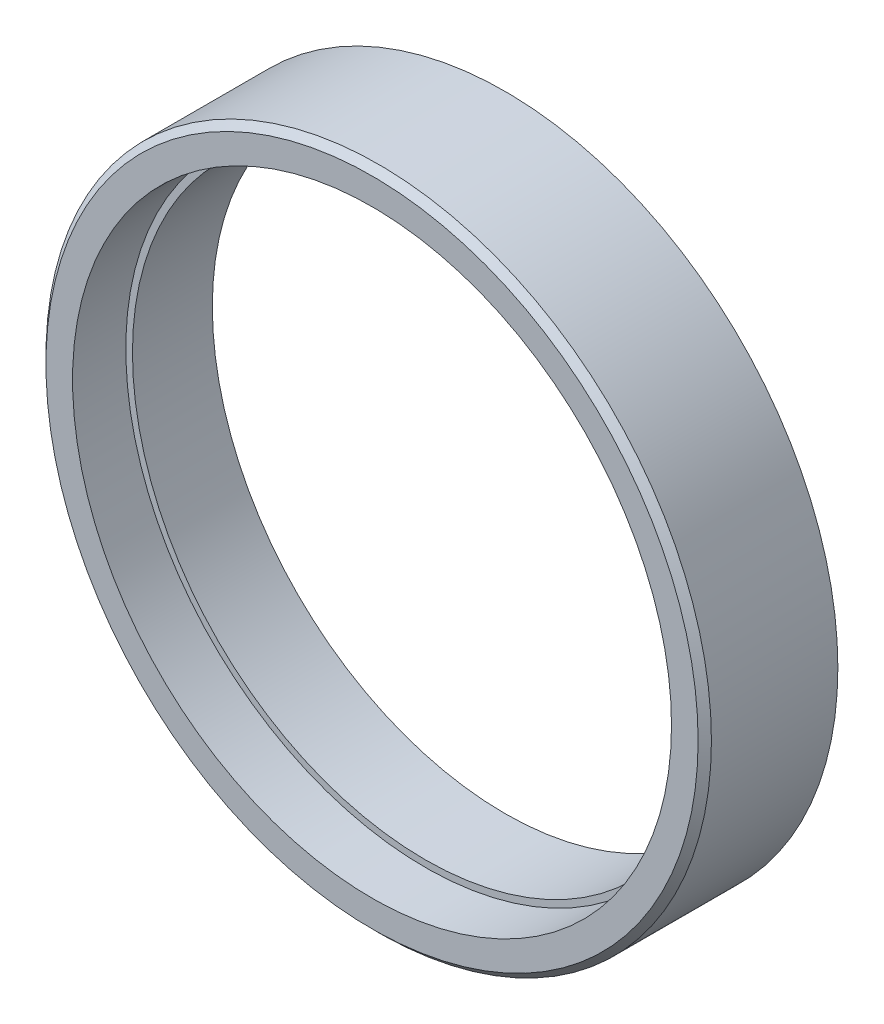
SolidWorks part; units mm, degrees
material "Plain Carbon Steel"
ref_plane "Front Plane" through (0, 0, 0) normal (0, 0, 1) x (1, 0, 0)
ref_plane "Top Plane" through (0, 0, 0) normal (0, 1, 0) x (1, 0, 0)
ref_plane "Right Plane" through (0, 0, 0) normal (1, 0, 0) x (0, 0, -1)
sketch "Rim OD Sketch Ø100" plane through (0, 0, 0) normal (0, 0, 1) x (1, 0, 0)
  circle A0 centre (0, 0) radius 50
  dimension "D1" = 100
extrude "Rim Blank Ø100x20" add sketch "Rim OD Sketch Ø100" along normal blind 20
sketch "Recess Sketch Ø90" plane through (0, 0, 20) normal (0, 0, 1) x (1, 0, 0)
  circle A0 centre (0, 0) radius 45
  dimension "D1" = 90
extrude "Recess Ø90x8" cut sketch "Recess Sketch Ø90" against normal blind 8
sketch "Bore Sketch Ø88" plane through (0, 0, 12) normal (0, 0, 1) x (1, 0, 0)
  circle A0 centre (0, 0) radius 44
  dimension "D1" = 88
extrude "Bore Ø88 Through" cut sketch "Bore Sketch Ø88" against normal blind 50
chamfer "Edge Chamfer 1x45deg" distance 1 angle 45 1 edges at (50, 0, 20)
